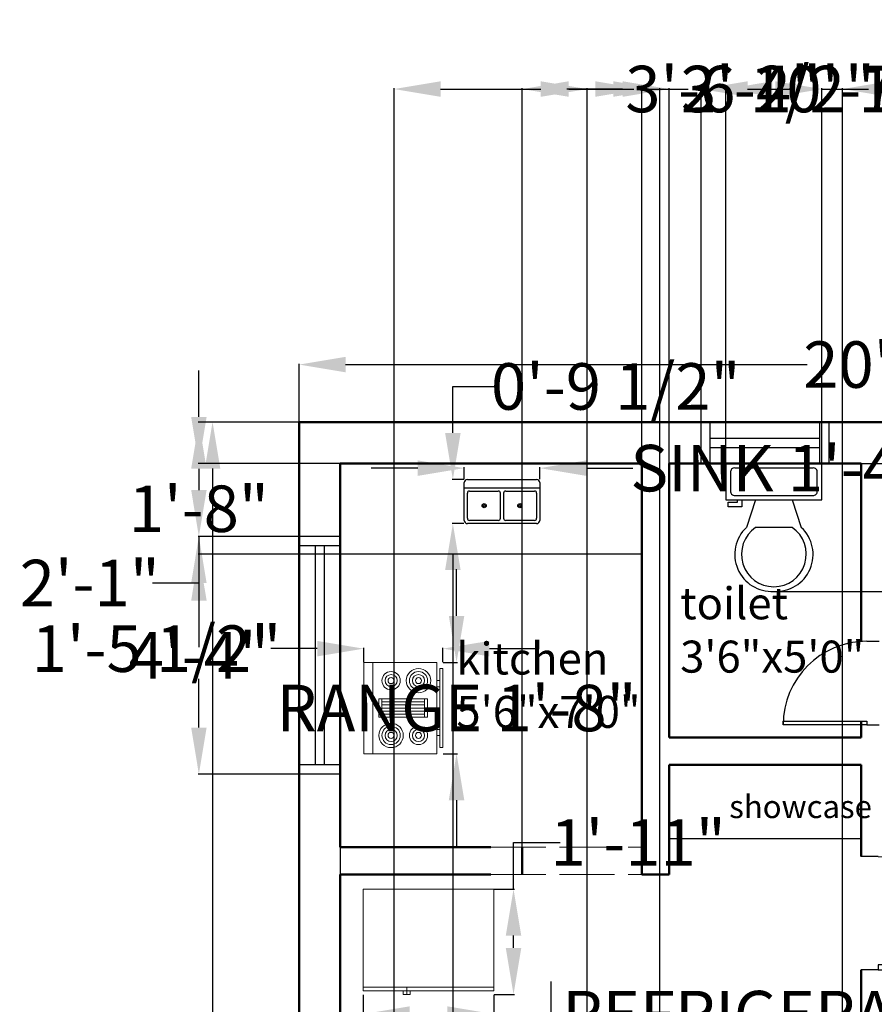
# Model space of a CAD drawing. Units: inches. Extents: x 19 to 1371, y 7 to 588.
# Tile 3 of 5: x 905 to 1092, y 372 to 588. Entities that reach past the tile are written whole.
import ezdxf

# ---------------------------------------------------------------- set-up
doc = ezdxf.new("R2010")
doc.units = ezdxf.units.IN
doc.header["$MEASUREMENT"] = 0
doc.linetypes.add('ACAD_ISO02W100', pattern=[15, 12, -3])
for name, color, linetype, lineweight in [('A-ANNO-DIMS', 2, 'Continuous', 18), ('A-ANNO-TEXT', 7, 'Continuous', 18), ('A-AREA-IDEN', 7, 'Continuous', 18), ('A-DOOR', 3, 'Continuous', 25), ('A-EQPM', 8, 'Continuous', 18), ('A-FLOR-CABN', 8, 'Continuous', 25), ('A-FLOR-FIXT', 9, 'Continuous', 25), ('A-GLAZ', 4, 'Continuous', 25), ('A-WALL', 7, 'Continuous', 50), ('A-WALL-OVHD', 8, 'ACAD_ISO02W100', 18)]:
    doc.layers.add(name, color=color, linetype=linetype, lineweight=lineweight)
doc.styles.get("Standard").update_dxf_attribs({"font": 'arial.ttf'})
doc.dimstyles.get("Standard").update_dxf_attribs({"dimtxt": 10.18, "dimasz": 10.18, "dimexe": 0.18, "dimexo": 0.0625, "dimgap": 0.09, "dimtad": 0, "dimtih": 1, "dimtoh": 1, "dimdec": 0, "dimzin": 0, "dimdsep": 46, "dimlunit": 3, "dimtxsty": 'Standard', "dimcen": 0.09, "dimadec": 0, "dimazin": 0, "dimtfac": 1, "dimtdec": 0, "dimtofl": 0, "dimtmove": 0, "dimatfit": 3, "dimfxl": 1, "dimtolj": 1, "dimtzin": 0, "dimarcsym": 0})

# ---------------------------------------------------------------- blocks, each defined once
blk = doc.blocks.new('*U2')
for p, q in [((0, 0), (0, -6)), ((40, 0), (40, -6))]:
    blk.add_line(p, q)
blk.add_lwpolyline([(0, 0), (0, 40), (1.75, 40), (1.75, 0)], close=True)
blk.add_arc((0, 0), 40, 0, 90)
blk = doc.blocks.new('*U4')
for p, q in [((9.5, -6), (9.5, -2)), ((-10, -8.5), (-8, -8.5)), ((-10, -9.5), (-10, -8.5)), ((-8, -8.5), (-8, -8)), ((-7, -8), (-7, -9.5)), ((-4, -8), (-6, -14)), ((4, -8), (6, -14)), ((-7, -9.5), (-10, -9.5)), ((4, -14), (-4, -14))]:
    blk.add_line(p, q)
blk.add_lwpolyline([(10.5, -8), (10.5, 0), (-10.5, 0), (-10.5, -8)], close=True)
for points in [[(-9.5, -2), (-9.5, -6)], [(8.5, -1), (-8.5, -1)], [(-8.5, -7), (8.5, -7)]]:
    blk.add_lwpolyline(points)
for centre, radius, start, end in [((-8.625, -1.875), 0.8839, 81.8699, 188.1301), ((8.625, -1.875), 0.8839, 351.8699, 98.1301), ((-8.625, -6.125), 0.8839, 171.869898, 278.1301), ((8.625, -6.125), 0.8839, 261.8699, 8.1301), ((-0.4772, -19.9188), 8.0953, 133.01722, 273.38), ((0.0374, -19.8731), 7.127, 124.50543, 269.7), ((-0.0373, -19.8731), 7.127, 270.3, 55.4946), ((0.4773, -19.9188), 8.0953, 266.62, 46.9828)]:
    blk.add_arc(centre, radius, start, end)
blk = doc.blocks.new('Sink-double - 36 in top')
for p, q in [((-18, -4), (18, -4)), ((-0.75, -18.5), (-0.75, -6.5)), ((0.75, -6.5), (0.75, -18.5))]:
    blk.add_line(p, q)
for points in [[(-16.5, 0), (16.5, 0)], [(-18, -19.5), (-18, -1.5)], [(18, -1.5), (18, -19.5)], [(-16.5, -18.5), (-16.5, -6.5)], [(-15.5, -5.5), (-1.75, -5.5)], [(1.75, -5.5), (15.5, -5.5)], [(16.5, -6.5), (16.5, -18.5)], [(16.5, -21), (-16.5, -21)], [(-1.75, -19.5), (-15.5, -19.5)], [(15.5, -19.5), (1.75, -19.5)]]:
    blk.add_lwpolyline(points)
for centre, radius in [((-8.5, -12.5), 1), ((-8.5, -12.5), 0.5), ((8.5, -12.5), 1), ((8.5, -12.5), 0.5)]:
    blk.add_circle(centre, radius)
for centre, radius, start, end in [((-16.5, -1.5), 1.5, 90, 180), ((16.5, -1.5), 1.5, 0, 90), ((-15.5, -6.5), 1, 90, 180), ((-1.75, -6.5), 1, 0, 90), ((1.75, -6.5), 1, 90, 180), ((15.5, -6.5), 1, 0, 90), ((-15.5, -18.5), 1, 180, 270), ((-1.75, -18.5), 1, 270, 0), ((1.75, -18.5), 1, 180, 270), ((15.5, -18.5), 1, 270, 0), ((-16.5, -19.5), 1.5, 180, 270), ((16.5, -19.5), 1.5, 270, 0)]:
    blk.add_arc(centre, radius, start, end)
blk = doc.blocks.new('Range-Oven - 30 in top')
for p, q in [((0, -3), (30, -3)), ((12, -6), (18, -6)), ((13, -20), (13, -6)), ((14, -6), (14, -20)), ((15, -20), (15, -6)), ((16, -6), (16, -20)), ((17, -20), (17, -6)), ((18, -20), (12, -20)), ((6, -24), (6, -25)), ((8, -25), (8, -24)), ((22, -25), (22, -24)), ((24, -24), (24, -25))]:
    blk.add_line(p, q)
for points in [[(0, -24), (0, 0), (30, 0), (30, -24)], [(12, -21), (12, -5), (18, -5), (18, -21)], [(2, -26), (2, -25), (28, -25), (28, -26)]]:
    blk.add_lwpolyline(points, close=True)
for centre, radius in [((6, -9), 4), ((6, -9), 3), ((24, -9), 3), ((6, -9), 2), ((6, -9), 1), ((24, -9), 2), ((24, -9), 1), ((6, -18), 3), ((6, -18), 2), ((24, -18), 4), ((24, -18), 3), ((24, -18), 2), ((6, -18), 1), ((24, -18), 1)]:
    blk.add_circle(centre, radius)
blk = doc.blocks.new('Refrigerator-2 door - 36 in top')
for p, q in [((0, -26.999999), (36, -26.999999)), ((12, -26.999999), (12, -28.999999)), ((11, -27.999999), (11, -28.999999)), ((11, -28.999999), (13, -28.999999)), ((13, -28.999999), (13, -27.999999))]:
    blk.add_line(p, q)
blk.add_lwpolyline([(0, -27.999999), (0, 0), (36, 0), (36, -27.999999)], close=True)
blk = doc.blocks.new('*D13')
at = {"layer": 'A-ANNO-DIMS', "color": 0, "lineweight": -2, "transparency": 16777216}
for p, q in [((966.44, 499.95), (966.44, 512.71)), ((976.62, 512.53), (1077.63, 512.53)), ((1196.26, 512.53), (1095.26, 512.53)), ((1206.44, 499.95), (1206.44, 512.71))]:
    blk.add_line(p, q, dxfattribs=at)
at = {"layer": 'A-ANNO-DIMS', "color": 0, "transparency": 16777216}
for points in [[(976.62, 514.22), (976.62, 510.83), (966.44, 512.53)], [(1196.26, 514.22), (1196.26, 510.83), (1206.44, 512.53)]]:
    blk.add_solid(points, dxfattribs=at)
at = {"layer": 'Defpoints', "color": 0, "transparency": 16777216}
for p in [(1206.44, 512.53), (966.44, 499.89), (1206.44, 499.89)]:
    blk.add_point(p, dxfattribs=at)
at = {"layer": 'A-ANNO-DIMS', "color": 0, "transparency": 16777216, "insert": (1086.44, 512.53), "char_height": 10.18, "attachment_point": 5}
blk.add_mtext("\\A1;20'", dxfattribs=at)
blk = doc.blocks.new('*D14')
at = {"layer": 'A-ANNO-DIMS', "color": 0, "lineweight": -2, "transparency": 16777216}
for p, q in [((966.38, 499.95), (947.31, 499.95)), ((947.49, 489.77), (947.49, 325.21)), ((947.49, 150.07), (947.49, 314.63)), ((966.38, 139.89), (947.31, 139.89))]:
    blk.add_line(p, q, dxfattribs=at)
at = {"layer": 'A-ANNO-DIMS', "color": 0, "transparency": 16777216}
for points in [[(945.79, 489.77), (949.18, 489.77), (947.49, 499.95)], [(945.79, 150.07), (949.18, 150.07), (947.49, 139.89)]]:
    blk.add_solid(points, dxfattribs=at)
at = {"layer": 'Defpoints', "color": 0, "transparency": 16777216}
for p in [(966.44, 499.95), (947.49, 139.89), (966.44, 139.89)]:
    blk.add_point(p, dxfattribs=at)
at = {"layer": 'A-ANNO-DIMS', "color": 0, "transparency": 16777216, "insert": (947.49, 319.92), "char_height": 10.18, "attachment_point": 5}
blk.add_mtext("\\A1;30'", dxfattribs=at)
blk = doc.blocks.new('WIN-24')
for p, q in [((0, 0), (0, 9)), ((2, 0), (2, 9)), ((26, 0), (26, 9)), ((28, 0), (28, 9)), ((2, 5.5), (26, 5.5)), ((2, 3.5), (26, 3.5))]:
    blk.add_line(p, q)
blk = doc.blocks.new('*D32')
at = {"layer": 'A-ANNO-DIMS', "color": 0, "lineweight": -2, "transparency": 16777216}
for p, q in [((992.39, 489.86), (982.21, 489.86)), ((1002.57, 487.44), (1002.57, 490.04)), ((1019.13, 487.44), (1019.13, 490.04)), ((1029.31, 489.86), (1039.49, 489.86))]:
    blk.add_line(p, q, dxfattribs=at)
at = {"layer": 'A-ANNO-DIMS', "color": 0, "transparency": 16777216}
for points in [[(992.39, 491.56), (992.39, 488.17), (1002.57, 489.86)], [(1029.31, 491.56), (1029.31, 488.17), (1019.13, 489.86)]]:
    blk.add_solid(points, dxfattribs=at)
at = {"layer": 'Defpoints', "color": 0, "transparency": 16777216}
for p in [(1019.13, 489.86), (1002.57, 487.38), (1019.13, 487.38)]:
    blk.add_point(p, dxfattribs=at)
at = {"layer": 'A-ANNO-DIMS', "color": 0, "transparency": 16777216, "insert": (1083.52, 489.86), "char_height": 10.18, "attachment_point": 5}
blk.add_mtext('\\A1;SINK 1\'-4 1/2"', dxfattribs=at)
blk = doc.blocks.new('*D33')
at = {"layer": 'A-ANNO-DIMS', "color": 0, "lineweight": -2, "transparency": 16777216}
for p, q in [((1000.09, 497.56), (1000.09, 507.74)), ((1000.09, 507.74), (1010.27, 507.74)), ((1002.51, 487.38), (999.91, 487.38)), ((1002.51, 477.72), (999.91, 477.72)), ((1000.09, 467.54), (1000.09, 457.36))]:
    blk.add_line(p, q, dxfattribs=at)
at = {"layer": 'A-ANNO-DIMS', "color": 0, "transparency": 16777216}
for points in [[(998.39, 497.56), (1001.79, 497.56), (1000.09, 487.38)], [(998.39, 467.54), (1001.79, 467.54), (1000.09, 477.72)]]:
    blk.add_solid(points, dxfattribs=at)
at = {"layer": 'Defpoints', "color": 0, "transparency": 16777216}
for p in [(1000.09, 487.38), (1002.57, 487.38), (1002.57, 477.72)]:
    blk.add_point(p, dxfattribs=at)
at = {"layer": 'A-ANNO-DIMS', "color": 0, "transparency": 16777216, "insert": (1035.75, 507.74), "char_height": 10.18, "attachment_point": 5}
blk.add_mtext('\\A1;0\'-9 1/2"', dxfattribs=at)
blk = doc.blocks.new('*D34')
at = {"layer": 'A-ANNO-DIMS', "color": 0, "lineweight": -2, "transparency": 16777216}
for p, q in [((1000.9, 457.53), (1000.9, 467.71)), ((997.96, 447.35), (1001.08, 447.35)), ((997.96, 427.35), (1001.08, 427.35)), ((1000.9, 417.17), (1000.9, 406.99))]:
    blk.add_line(p, q, dxfattribs=at)
at = {"layer": 'A-ANNO-DIMS', "color": 0, "transparency": 16777216}
for points in [[(999.2, 457.53), (1002.6, 457.53), (1000.9, 447.35)], [(999.2, 417.17), (1002.6, 417.17), (1000.9, 427.35)]]:
    blk.add_solid(points, dxfattribs=at)
at = {"layer": 'Defpoints', "color": 0, "transparency": 16777216}
for p in [(997.9, 447.35), (1000.9, 447.35), (997.9, 427.35)]:
    blk.add_point(p, dxfattribs=at)
at = {"layer": 'A-ANNO-DIMS', "color": 0, "transparency": 16777216, "insert": (1000.9, 437.35), "char_height": 10.18, "attachment_point": 5}
blk.add_mtext('\\A1;RANGE 1\'-8"', dxfattribs=at)
blk = doc.blocks.new('*D35')
at = {"layer": 'A-ANNO-DIMS', "color": 0, "lineweight": -2, "transparency": 16777216}
for p, q in [((980.57, 447.41), (980.57, 450.53)), ((997.9, 447.41), (997.9, 450.53)), ((970.39, 450.35), (960.21, 450.35)), ((1008.08, 450.35), (1018.26, 450.35))]:
    blk.add_line(p, q, dxfattribs=at)
at = {"layer": 'A-ANNO-DIMS', "color": 0, "transparency": 16777216}
for points in [[(970.39, 452.04), (970.39, 448.65), (980.57, 450.35)], [(1008.08, 452.04), (1008.08, 448.65), (997.9, 450.35)]]:
    blk.add_solid(points, dxfattribs=at)
at = {"layer": 'Defpoints', "color": 0, "transparency": 16777216}
for p in [(980.57, 450.35), (980.57, 447.35), (997.9, 447.35)]:
    blk.add_point(p, dxfattribs=at)
at = {"layer": 'A-ANNO-DIMS', "color": 0, "transparency": 16777216, "insert": (935.21, 450.35), "char_height": 10.18, "attachment_point": 5}
blk.add_mtext('\\A1;1\'-5 1/2"', dxfattribs=at)
blk = doc.blocks.new('*D36')
at = {"layer": 'A-ANNO-DIMS', "color": 0, "lineweight": -2, "transparency": 16777216}
for p, q in [((980.44, 374.59), (980.44, 370.17)), ((1009.08, 374.59), (1009.08, 370.17)), ((990.62, 370.35), (998.9, 370.35)), ((1009.08, 370.35), (1019.26, 370.35))]:
    blk.add_line(p, q, dxfattribs=at)
at = {"layer": 'A-ANNO-DIMS', "color": 0, "transparency": 16777216}
for points in [[(990.62, 372.05), (990.62, 368.66), (980.44, 370.35)], [(998.9, 372.05), (998.9, 368.66), (1009.08, 370.35)]]:
    blk.add_solid(points, dxfattribs=at)
at = {"layer": 'Defpoints', "color": 0, "transparency": 16777216}
for p in [(980.44, 374.65), (1009.08, 374.65), (1009.08, 370.35)]:
    blk.add_point(p, dxfattribs=at)
at = {"layer": 'A-ANNO-DIMS', "color": 0, "transparency": 16777216, "insert": (1102.94, 370.35), "char_height": 10.18, "attachment_point": 5}
blk.add_mtext('\\A1;REFRIGERATOR 2\'-4 1/2"', dxfattribs=at)
blk = doc.blocks.new('*D37')
at = {"layer": 'A-ANNO-DIMS', "color": 0, "lineweight": -2, "transparency": 16777216}
for p, q in [((1013.37, 397.72), (1013.37, 407.9)), ((1013.37, 407.9), (1023.55, 407.9)), ((1009.14, 397.72), (1013.55, 397.72)), ((1013.37, 384.83), (1013.37, 387.54)), ((1009.14, 374.65), (1013.55, 374.65))]:
    blk.add_line(p, q, dxfattribs=at)
at = {"layer": 'A-ANNO-DIMS', "color": 0, "transparency": 16777216}
for points in [[(1011.68, 387.54), (1015.07, 387.54), (1013.37, 397.72)], [(1011.68, 384.83), (1015.07, 384.83), (1013.37, 374.65)]]:
    blk.add_solid(points, dxfattribs=at)
at = {"layer": 'Defpoints', "color": 0, "transparency": 16777216}
for p in [(1009.08, 397.72), (1013.37, 397.72), (1009.08, 374.65)]:
    blk.add_point(p, dxfattribs=at)
at = {"layer": 'A-ANNO-DIMS', "color": 0, "transparency": 16777216, "insert": (1040.65, 407.9), "char_height": 10.18, "attachment_point": 5}
blk.add_mtext('\\A1;1\'-11"', dxfattribs=at)
blk = doc.blocks.new('*D39')
at = {"layer": 'A-ANNO-DIMS', "color": 0, "lineweight": -2, "transparency": 16777216}
for p, q in [((1021.61, 367.32), (1021.61, 377.5)), ((1017.55, 357.14), (1021.79, 357.14)), ((1017.55, 340.54), (1021.79, 340.54)), ((1021.61, 330.36), (1021.61, 320.18))]:
    blk.add_line(p, q, dxfattribs=at)
at = {"layer": 'A-ANNO-DIMS', "color": 0, "transparency": 16777216}
for points in [[(1019.91, 367.32), (1023.31, 367.32), (1021.61, 357.14)], [(1019.91, 330.36), (1023.31, 330.36), (1021.61, 340.54)]]:
    blk.add_solid(points, dxfattribs=at)
at = {"layer": 'Defpoints', "color": 0, "transparency": 16777216}
for p in [(1017.49, 357.14), (1021.61, 357.14), (1017.49, 340.54)]:
    blk.add_point(p, dxfattribs=at)
at = {"layer": 'A-ANNO-DIMS', "color": 0, "transparency": 16777216, "insert": (1021.61, 348.84), "char_height": 10.18, "attachment_point": 5}
blk.add_mtext('\\A1;1\'-4 1/2"', dxfattribs=at)
blk = doc.blocks.new('*D46')
at = {"layer": 'A-ANNO-DIMS', "color": 0, "lineweight": -2, "transparency": 16777216}
for p, q in [((1035.21, 572.84), (1025.03, 572.84)), ((1045.39, 211.95), (1045.39, 573.02)), ((1085.39, 211.95), (1085.39, 573.02)), ((1095.57, 572.84), (1105.75, 572.84))]:
    blk.add_line(p, q, dxfattribs=at)
at = {"layer": 'A-ANNO-DIMS', "color": 0, "transparency": 16777216}
for points in [[(1035.21, 574.54), (1035.21, 571.14), (1045.39, 572.84)], [(1095.57, 574.54), (1095.57, 571.14), (1085.39, 572.84)]]:
    blk.add_solid(points, dxfattribs=at)
at = {"layer": 'Defpoints', "color": 0, "transparency": 16777216}
for p in [(1085.39, 572.84), (1045.39, 211.89), (1085.39, 211.89)]:
    blk.add_point(p, dxfattribs=at)
at = {"layer": 'A-ANNO-DIMS', "color": 0, "transparency": 16777216, "insert": (1065.39, 572.84), "char_height": 10.18, "attachment_point": 5}
blk.add_mtext('\\A1;3\'-4"', dxfattribs=at)
blk = doc.blocks.new('*D47')
at = {"layer": 'A-ANNO-DIMS', "color": 0, "lineweight": -2, "transparency": 16777216}
for p, q in [((987.23, 211.95), (987.23, 573.02)), ((997.41, 572.84), (1019.34, 572.84)), ((1029.52, 211.95), (1029.52, 573.02)), ((1029.52, 572.84), (1039.7, 572.84))]:
    blk.add_line(p, q, dxfattribs=at)
at = {"layer": 'A-ANNO-DIMS', "color": 0, "transparency": 16777216}
for points in [[(997.41, 574.54), (997.41, 571.14), (987.23, 572.84)], [(1019.34, 574.54), (1019.34, 571.14), (1029.52, 572.84)]]:
    blk.add_solid(points, dxfattribs=at)
at = {"layer": 'Defpoints', "color": 0, "transparency": 16777216}
for p in [(1029.52, 572.84), (987.23, 211.89), (1029.52, 211.89)]:
    blk.add_point(p, dxfattribs=at)
at = {"layer": 'A-ANNO-DIMS', "color": 0, "transparency": 16777216, "insert": (1065.17, 572.84), "char_height": 10.18, "attachment_point": 5}
blk.add_mtext('\\A1;3\'-6 1/2"', dxfattribs=at)
blk = doc.blocks.new('*D55')
at = {"layer": 'A-ANNO-DIMS', "color": 0, "lineweight": -2, "transparency": 16777216}
for p, q in [((944.49, 501.07), (944.49, 511.25)), ((1041.38, 490.89), (944.31, 490.89)), ((1041.38, 471.04), (944.31, 471.04)), ((944.49, 460.86), (944.49, 450.68))]:
    blk.add_line(p, q, dxfattribs=at)
at = {"layer": 'A-ANNO-DIMS', "color": 0, "transparency": 16777216}
for points in [[(942.8, 501.07), (946.19, 501.07), (944.49, 490.89)], [(942.8, 460.86), (946.19, 460.86), (944.49, 471.04)]]:
    blk.add_solid(points, dxfattribs=at)
at = {"layer": 'Defpoints', "color": 0, "transparency": 16777216}
for p in [(944.49, 490.89), (1041.44, 490.89), (1041.44, 471.04)]:
    blk.add_point(p, dxfattribs=at)
at = {"layer": 'A-ANNO-DIMS', "color": 0, "transparency": 16777216, "insert": (944.49, 480.97), "char_height": 10.18, "attachment_point": 5}
blk.add_mtext('\\A1;1\'-8"', dxfattribs=at)
blk = doc.blocks.new('*D56')
at = {"layer": 'A-ANNO-DIMS', "color": 0, "lineweight": -2, "transparency": 16777216}
for p, q in [((975.44, 406.83), (975.44, 117.76)), ((1000.05, 406.83), (1000.05, 117.76)), ((985.62, 117.94), (989.87, 117.94)), ((1000.05, 117.94), (1010.23, 117.94))]:
    blk.add_line(p, q, dxfattribs=at)
at = {"layer": 'A-ANNO-DIMS', "color": 0, "transparency": 16777216}
for points in [[(985.62, 119.64), (985.62, 116.24), (975.44, 117.94)], [(989.87, 119.64), (989.87, 116.24), (1000.05, 117.94)]]:
    blk.add_solid(points, dxfattribs=at)
at = {"layer": 'Defpoints', "color": 0, "transparency": 16777216}
for p in [(975.44, 406.89), (1000.05, 406.89), (1000.05, 117.94)]:
    blk.add_point(p, dxfattribs=at)
at = {"layer": 'A-ANNO-DIMS', "color": 0, "transparency": 16777216, "insert": (1035.8, 117.94), "char_height": 10.18, "attachment_point": 5}
blk.add_mtext('\\A1;2\'-0 1/2"', dxfattribs=at)
blk = doc.blocks.new('*D57')
at = {"layer": 'A-ANNO-DIMS', "color": 0, "lineweight": -2, "transparency": 16777216}
for p, q in [((966.38, 499.89), (944.31, 499.89)), ((944.49, 489.71), (944.49, 485.07)), ((966.38, 474.89), (944.31, 474.89)), ((944.49, 474.89), (944.49, 464.71)), ((944.49, 464.71), (934.31, 464.71))]:
    blk.add_line(p, q, dxfattribs=at)
at = {"layer": 'A-ANNO-DIMS', "color": 0, "transparency": 16777216}
for points in [[(942.8, 489.71), (946.19, 489.71), (944.49, 499.89)], [(942.8, 485.07), (946.19, 485.07), (944.49, 474.89)]]:
    blk.add_solid(points, dxfattribs=at)
at = {"layer": 'Defpoints', "color": 0, "transparency": 16777216}
for p in [(966.44, 499.89), (944.49, 474.89), (966.44, 474.89)]:
    blk.add_point(p, dxfattribs=at)
at = {"layer": 'A-ANNO-DIMS', "color": 0, "transparency": 16777216, "insert": (920.61, 464.71), "char_height": 10.18, "attachment_point": 5}
blk.add_mtext('\\A1;2\'-1"', dxfattribs=at)
blk = doc.blocks.new('*D58')
at = {"layer": 'A-ANNO-DIMS', "color": 0, "lineweight": -2, "transparency": 16777216}
for p, q in [((966.38, 474.89), (944.31, 474.89)), ((944.49, 464.71), (944.49, 454.07)), ((944.49, 433.07), (944.49, 443.71)), ((966.38, 422.89), (944.31, 422.89))]:
    blk.add_line(p, q, dxfattribs=at)
at = {"layer": 'A-ANNO-DIMS', "color": 0, "transparency": 16777216}
for points in [[(942.8, 464.71), (946.19, 464.71), (944.49, 474.89)], [(942.8, 433.07), (946.19, 433.07), (944.49, 422.89)]]:
    blk.add_solid(points, dxfattribs=at)
at = {"layer": 'Defpoints', "color": 0, "transparency": 16777216}
for p in [(944.49, 474.89), (966.44, 474.89), (966.44, 422.89)]:
    blk.add_point(p, dxfattribs=at)
at = {"layer": 'A-ANNO-DIMS', "color": 0, "transparency": 16777216, "insert": (944.49, 448.89), "char_height": 10.18, "attachment_point": 5}
blk.add_mtext('\\A1;4\'-4"', dxfattribs=at)
blk = doc.blocks.new('*D64')
at = {"layer": 'A-ANNO-DIMS', "color": 0, "lineweight": -2, "transparency": 16777216}
for p, q in [((1037.26, 572.84), (1027.08, 572.84)), ((1047.44, 490.95), (1047.44, 573.02)), ((1054.44, 490.95), (1054.44, 573.02)), ((1064.62, 572.84), (1074.8, 572.84))]:
    blk.add_line(p, q, dxfattribs=at)
at = {"layer": 'A-ANNO-DIMS', "color": 0, "transparency": 16777216}
for points in [[(1037.26, 574.54), (1037.26, 571.14), (1047.44, 572.84)], [(1064.62, 574.54), (1064.62, 571.14), (1054.44, 572.84)]]:
    blk.add_solid(points, dxfattribs=at)
at = {"layer": 'Defpoints', "color": 0, "transparency": 16777216}
for p in [(1054.44, 572.84), (1047.44, 490.89), (1054.44, 490.89)]:
    blk.add_point(p, dxfattribs=at)
at = {"layer": 'A-ANNO-DIMS', "color": 0, "transparency": 16777216, "insert": (1088.42, 572.84), "char_height": 10.18, "attachment_point": 5}
blk.add_mtext('\\A1;0\'-7"', dxfattribs=at)
blk = doc.blocks.new('*D68')
at = {"layer": 'A-ANNO-DIMS', "color": 0, "lineweight": -2, "transparency": 16777216}
for p, q in [((1059.87, 490.95), (1059.87, 573.02)), ((1070.05, 572.84), (1070.69, 572.84)), ((1080.87, 490.95), (1080.87, 573.02)), ((1080.87, 572.84), (1091.05, 572.84))]:
    blk.add_line(p, q, dxfattribs=at)
at = {"layer": 'A-ANNO-DIMS', "color": 0, "transparency": 16777216}
for points in [[(1070.05, 574.54), (1070.05, 571.14), (1059.87, 572.84)], [(1070.69, 574.54), (1070.69, 571.14), (1080.87, 572.84)]]:
    blk.add_solid(points, dxfattribs=at)
at = {"layer": 'Defpoints', "color": 0, "transparency": 16777216}
for p in [(1080.87, 572.84), (1059.87, 490.89), (1080.87, 490.89)]:
    blk.add_point(p, dxfattribs=at)
at = {"layer": 'A-ANNO-DIMS', "color": 0, "transparency": 16777216, "insert": (1104.19, 572.84), "char_height": 10.18, "attachment_point": 5}
blk.add_mtext('\\A1;1\'-9"', dxfattribs=at)
blk = doc.blocks.new('*D69')
at = {"layer": 'A-ANNO-DIMS', "color": 0, "lineweight": -2, "transparency": 16777216}
for p, q in [((1080.93, 490.89), (1228.57, 490.89)), ((1228.39, 480.71), (1228.39, 473.07)), ((1070.43, 462.89), (1228.57, 462.89)), ((1228.39, 462.89), (1228.39, 452.71)), ((1228.39, 452.71), (1218.21, 452.71))]:
    blk.add_line(p, q, dxfattribs=at)
at = {"layer": 'A-ANNO-DIMS', "color": 0, "transparency": 16777216}
for points in [[(1226.7, 480.71), (1230.09, 480.71), (1228.39, 490.89)], [(1226.7, 473.07), (1230.09, 473.07), (1228.39, 462.89)]]:
    blk.add_solid(points, dxfattribs=at)
at = {"layer": 'Defpoints', "color": 0, "transparency": 16777216}
for p in [(1080.87, 490.89), (1070.37, 462.89), (1228.39, 462.89)]:
    blk.add_point(p, dxfattribs=at)
at = {"layer": 'A-ANNO-DIMS', "color": 0, "transparency": 16777216, "insert": (1204.51, 452.71), "char_height": 10.18, "attachment_point": 5}
blk.add_mtext('\\A1;2\'-4"', dxfattribs=at)
blk = doc.blocks.new('*D70')
at = {"layer": 'A-ANNO-DIMS', "color": 0, "lineweight": -2, "transparency": 16777216}
for p, q in [((1015.29, 400.95), (1015.29, 573.02)), ((1025.47, 572.84), (1031.26, 572.84)), ((1041.44, 400.95), (1041.44, 573.02)), ((1041.44, 572.84), (1051.62, 572.84))]:
    blk.add_line(p, q, dxfattribs=at)
at = {"layer": 'A-ANNO-DIMS', "color": 0, "transparency": 16777216}
for points in [[(1025.47, 574.54), (1025.47, 571.14), (1015.29, 572.84)], [(1031.26, 574.54), (1031.26, 571.14), (1041.44, 572.84)]]:
    blk.add_solid(points, dxfattribs=at)
at = {"layer": 'Defpoints', "color": 0, "transparency": 16777216}
for p in [(1041.44, 572.84), (1015.29, 400.89), (1041.44, 400.89)]:
    blk.add_point(p, dxfattribs=at)
at = {"layer": 'A-ANNO-DIMS', "color": 0, "transparency": 16777216, "insert": (1065.33, 572.84), "char_height": 10.18, "attachment_point": 5}
blk.add_mtext('\\A1;2\'-2"', dxfattribs=at)

msp = doc.modelspace()

# ---------------------------------------------------------------- linework, layer by layer
at = {"layer": 'A-FLOR-CABN'}
for p, q in [((1041.44, 471.04), (1000.05, 471.04)), ((1000.05, 471.04), (1000.05, 406.89)), ((1041.44, 471.04), (1041.44, 471.04)), ((1047.44, 408.8), (1089.44, 408.8))]:
    msp.add_line(p, q, dxfattribs=at)
at = {"layer": 'A-GLAZ'}
for p, q in [((975.44, 474.89), (966.44, 474.89)), ((975.44, 472.89), (966.44, 472.89)), ((969.94, 472.89), (969.94, 424.89)), ((971.94, 472.89), (971.94, 424.89)), ((971.94, 472.89), (971.94, 424.89)), ((971.94, 472.89), (971.94, 424.89)), ((975.44, 424.89), (966.44, 424.89)), ((975.44, 422.89), (966.44, 422.89))]:
    msp.add_line(p, q, dxfattribs=at)
at = {"layer": 'A-WALL'}
for p, q in [((966.44, 139.89), (966.44, 499.89)), ((966.44, 499.89), (1206.44, 499.89)), ((975.44, 490.89), (1041.44, 490.89)), ((975.44, 406.89), (975.44, 490.89)), ((1041.44, 406.89), (1041.44, 490.89)), ((1047.44, 430.89), (1047.44, 490.89)), ((1047.44, 490.89), (1089.44, 490.89)), ((1089.44, 451.92), (1089.44, 490.89)), ((1089.44, 430.89), (1089.44, 434.44)), ((1047.44, 430.89), (1089.44, 430.89)), ((1047.44, 424.89), (1089.44, 424.89)), ((1047.44, 400.89), (1047.44, 424.89)), ((1089.44, 404.87), (1089.44, 424.89)), ((975.44, 406.89), (1008.44, 406.89)), ((1015.29, 406.89), (1015.29, 400.89)), ((1041.44, 406.89), (1041.44, 400.89)), ((975.44, 148.89), (975.44, 400.89)), ((975.44, 400.89), (1008.44, 400.89)), ((1041.44, 400.89), (1047.44, 400.89)), ((1089.44, 355.24), (1089.44, 380.02))]:
    msp.add_line(p, q, dxfattribs=at)
at = {"layer": 'A-WALL-OVHD'}
for p, q in [((1008.44, 406.89), (1041.44, 406.89)), ((1008.44, 400.89), (1041.44, 400.89))]:
    msp.add_line(p, q, dxfattribs=at)

# ---------------------------------------------------------------- block references
at = {"layer": 'A-DOOR'}
for p, xscale, yscale, zscale, rotation in [((1090.69, 433.64), 0.4579245056729436, 0.4579245056729436, 0.4579245056729436, 90), ((1093.17, 380.02), -0.6212879094378088, 0.6212879094378088, 0.6212879094378088, 270)]:
    msp.add_blockref('*U2', p, dxfattribs=dict(at, xscale=xscale, yscale=yscale, zscale=zscale, rotation=rotation))
at = {"layer": 'A-EQPM', "xscale": 0.6666666080000113, "yscale": 0.6666666080000113, "zscale": 0.6666666080000113, "rotation": 90}
msp.add_blockref('Range-Oven - 30 in top', (980.57, 427.35), dxfattribs=at)
at = {"layer": 'A-EQPM', "xscale": 0.7954344782942591, "yscale": 0.7954344782942591, "zscale": 0.7954344782942591}
msp.add_blockref('Refrigerator-2 door - 36 in top', (980.44, 397.72), dxfattribs=at)
at = {"layer": 'A-FLOR-FIXT'}
msp.add_blockref('*U4', (1070.37, 490.89), dxfattribs=at)
at = {"layer": 'A-FLOR-FIXT', "xscale": 0.4598112006574885, "yscale": 0.4598112006574885, "zscale": 0.4598112006574885}
msp.add_blockref('Sink-double - 36 in top', (1010.85, 487.38), dxfattribs=at)
at = {"layer": 'A-GLAZ'}
msp.add_blockref('WIN-24', (1054.44, 490.89), dxfattribs=at)

# ---------------------------------------------------------------- texts
at = {"layer": 'A-ANNO-TEXT', "insert": (1060.59, 418.26), "char_height": 5, "attachment_point": 1}
msp.add_mtext_dynamic_manual_height_columns('showcase', width=24.0321, gutter_width=1, heights=[0], dxfattribs=at)
at = {"layer": 'A-AREA-IDEN', "char_height": 7, "attachment_point": 1}
for s, insert in [('toilet\\P3\'6"x5\'0"', (1049.85, 463.77)), ('kitchen\\P5\'6"x7\'0"', (1000.86, 451.68))]:
    msp.add_mtext_dynamic_manual_height_columns(s, width=53.7683, gutter_width=1, heights=[0], dxfattribs=dict(at, insert=insert))

# ---------------------------------------------------------------- dimensions: what is measured, and where the dimension line sits
at = {"layer": 'A-ANNO-DIMS'}
for base, p1, p2, override, picture, middle in [((1029.52, 572.84), (987.23, 211.89), (1029.52, 211.89), {"dimdec": 1, "dimlfac": 1, "dimrnd": 0, "dimzin": 1, "dimdsep": 46, "dimlunit": 4, "dimfrac": 2}, '*D47', (1065.17, 572.84)), ((1041.4425, 572.8408), (1015.289, 400.8908), (1041.4425, 400.8908), {"dimdec": 1, "dimlfac": 1, "dimrnd": 0, "dimzin": 1, "dimdsep": 46, "dimlunit": 4, "dimfrac": 2}, '*D70', (1065.3298, 572.8408)), ((1085.39, 572.84), (1045.39, 211.89), (1085.39, 211.89), {"dimdec": 1, "dimlfac": 1, "dimrnd": 0, "dimzin": 1, "dimdsep": 46, "dimlunit": 4, "dimfrac": 2}, '*D46', (1065.39, 572.84)), ((1054.44, 572.84), (1047.44, 490.89), (1054.44, 490.89), {"dimdec": 1, "dimlfac": 1, "dimrnd": 0, "dimzin": 1, "dimdsep": 46, "dimlunit": 4, "dimfrac": 2}, '*D64', (1088.42, 572.84)), ((1080.87, 572.84), (1059.87, 490.89), (1080.87, 490.89), {"dimdec": 1, "dimlfac": 1, "dimrnd": 0, "dimzin": 1, "dimdsep": 46, "dimlunit": 4, "dimfrac": 2}, '*D68', (1104.19, 572.84)), ((1206.44, 512.53), (966.44, 499.89), (1206.44, 499.89), {"dimclrd": 0, "dimclre": 0, "dimclrt": 0}, '*D13', (1086.44, 512.53)), ((1000.05, 117.94), (975.44, 406.89), (1000.05, 406.89), {"dimdec": 1, "dimlfac": 1, "dimrnd": 0, "dimzin": 1, "dimdsep": 46, "dimlunit": 4, "dimfrac": 2}, '*D56', (1035.8, 117.94))]:
    dim = msp.add_linear_dim(base=base, p1=p1, p2=p2, dimstyle='Standard', override=override, dxfattribs=at)
    dim.commit()
    dim.dimension.update_dxf_attribs({"geometry": picture, "text_midpoint": middle})
for base, p1, p2, angle, override, picture, middle in [((1000.09, 487.38), (1002.57, 477.72), (1002.57, 487.38), 90, {"dimdec": 1, "dimlfac": 1, "dimrnd": 0, "dimzin": 1, "dimdsep": 46, "dimlunit": 4, "dimfrac": 2}, '*D33', (1035.75, 507.74)), ((944.4925, 490.8908), (1041.4425, 471.0399), (1041.4425, 490.8908), 90, {"dimdec": 1, "dimlfac": 1, "dimrnd": 0, "dimzin": 1, "dimdsep": 46, "dimlunit": 4, "dimfrac": 2}, '*D55', (944.4925, 480.9654)), ((944.49, 474.89), (966.44, 499.89), (966.44, 474.89), 90, {"dimdec": 1, "dimlfac": 1, "dimrnd": 0, "dimzin": 1, "dimdsep": 46, "dimlunit": 4, "dimfrac": 2}, '*D57', (920.61, 464.71)), ((947.49, 139.89), (966.44, 499.95), (966.44, 139.89), 90, {"dimclrd": 0, "dimclre": 0, "dimclrt": 0}, '*D14', (947.49, 319.92)), ((1228.39, 462.89), (1080.87, 490.89), (1070.37, 462.89), 90, {"dimdec": 1, "dimlfac": 1, "dimrnd": 0, "dimzin": 1, "dimdsep": 46, "dimlunit": 4, "dimfrac": 2}, '*D69', (1204.51, 452.71)), ((944.49, 474.89), (966.44, 422.89), (966.44, 474.89), 90, {"dimdec": 1, "dimlfac": 1, "dimrnd": 0, "dimzin": 1, "dimdsep": 46, "dimlunit": 4, "dimfrac": 2}, '*D58', (944.49, 448.89)), ((980.57, 450.35), (997.9, 447.35), (980.57, 447.35), 180, {"dimdec": 1, "dimlfac": 1, "dimrnd": 0, "dimzin": 1, "dimdsep": 46, "dimlunit": 4, "dimfrac": 2}, '*D35', (935.21, 450.35)), ((1013.37, 397.72), (1009.08, 374.65), (1009.08, 397.72), 90, {"dimdec": 1, "dimlfac": 1, "dimrnd": 0, "dimzin": 1, "dimdsep": 46, "dimlunit": 4, "dimfrac": 2}, '*D37', (1040.65, 407.9)), ((1021.61, 357.14), (1017.49, 340.54), (1017.49, 357.14), 90, {"dimdec": 1, "dimlfac": 1, "dimrnd": 0, "dimzin": 1, "dimdsep": 46, "dimlunit": 4, "dimfrac": 2}, '*D39', (1021.61, 348.84))]:
    dim = msp.add_linear_dim(base=base, p1=p1, p2=p2, angle=angle, dimstyle='Standard', override=override, dxfattribs=at)
    dim.commit()
    dim.dimension.update_dxf_attribs({"geometry": picture, "text_midpoint": middle})
for base, p1, p2, text, picture, middle in [((1019.13, 489.86), (1002.57, 487.38), (1019.13, 487.38), 'SINK <>', '*D32', (1083.52, 489.86)), ((1009.08, 370.35), (980.44, 374.65), (1009.08, 374.65), 'REFRIGERATOR <>', '*D36', (1102.94, 370.35))]:
    dim = msp.add_linear_dim(base=base, p1=p1, p2=p2, text=text, dimstyle='Standard', override={"dimdec": 1, "dimlfac": 1, "dimrnd": 0, "dimzin": 1, "dimdsep": 46, "dimlunit": 4, "dimfrac": 2}, dxfattribs=at)
    dim.commit()
    dim.dimension.update_dxf_attribs({"geometry": picture, "text_midpoint": middle})
dim = msp.add_linear_dim(base=(1000.9, 447.35), p1=(997.9, 427.35), p2=(997.9, 447.35), angle=90, text='RANGE <>', dimstyle='Standard', override={"dimdec": 1, "dimlfac": 1, "dimrnd": 0, "dimzin": 1, "dimdsep": 46, "dimlunit": 4, "dimfrac": 2}, dxfattribs=at)
dim.commit()
dim.dimension.update_dxf_attribs({"geometry": '*D34', "text_midpoint": (1000.9, 437.35)})

doc.saveas('drawing.dxf')
